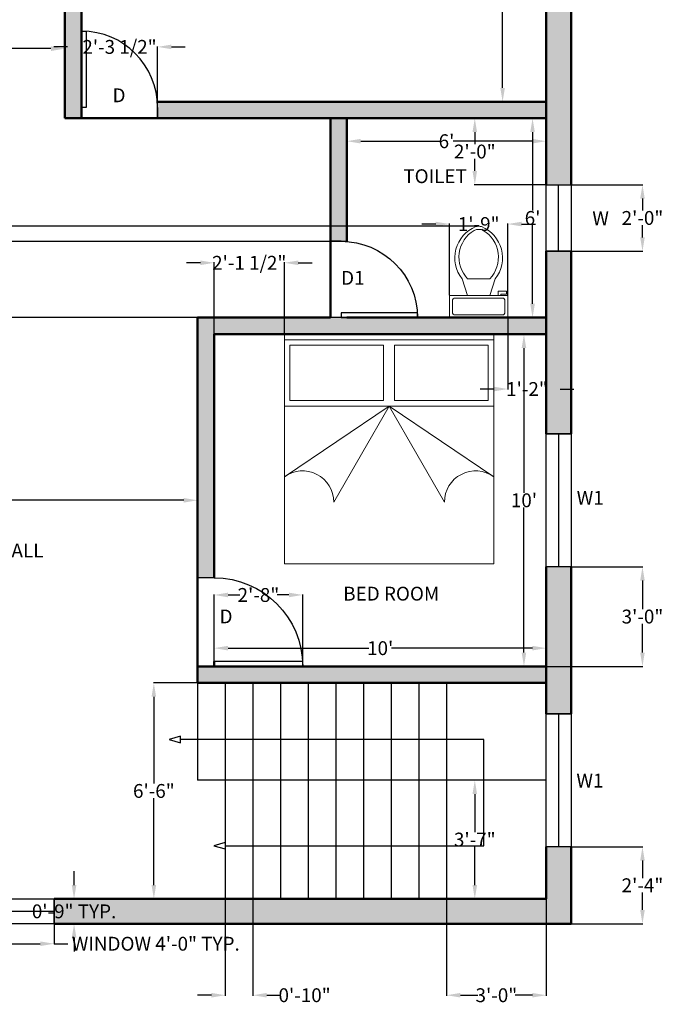
# Model space of a CAD drawing. Units: inches. Extents: x 3136 to 3620, y 13606 to 14152.
# Tile 5 of 6: x 3386 to 3618, y 13610 to 13965. Entities that reach past the tile are written whole.
import ezdxf

# ---------------------------------------------------------------- set-up
doc = ezdxf.new("R2010")
doc.units = ezdxf.units.IN
for name, color, linetype, lineweight in [('A-ANNO-DIMS', 2, 'Continuous', 18), ('A-ANNO-TEXT', 7, 'Continuous', 18), ('A-AREA-IDEN', 7, 'Continuous', 25), ('A-DOOR', 3, 'Continuous', 25), ('A-FLOR-FIXT', 9, 'Continuous', 18), ('A-FLOR-STRS', 7, 'Continuous', 25), ('A-FURN', 8, 'Continuous', 18), ('A-GLAZ', 4, 'Continuous', 25), ('A-WALL', 7, 'Continuous', 50), ('A-WALL-PATT', 174, 'Continuous', 13)]:
    doc.layers.add(name, color=color, linetype=linetype, lineweight=lineweight)
doc.styles.get("Standard").update_dxf_attribs({"font": 'arial.ttf', "height": 5})
doc.dimstyles.get("Standard").update_dxf_attribs({"dimtxt": 5, "dimasz": 5, "dimexe": 0.18, "dimexo": 0.0625, "dimgap": 0.09, "dimtad": 0, "dimtih": 1, "dimtoh": 1, "dimdec": 0, "dimzin": 0, "dimdsep": 46, "dimlunit": 3, "dimtxsty": 'Standard', "dimcen": 0.09, "dimadec": 0, "dimazin": 0, "dimtfac": 1, "dimtdec": 0, "dimtofl": 0, "dimtmove": 0, "dimatfit": 3, "dimfxl": 1, "dimtolj": 1, "dimtzin": 0, "dimarcsym": 0})

# ---------------------------------------------------------------- blocks, each defined once
blk = doc.blocks.new('*U4')
for p, q in [((0, 0), (0, -6)), ((32, 0), (32, -6))]:
    blk.add_line(p, q)
blk.add_lwpolyline([(0, 0), (0, 32), (1.75, 32), (1.75, 0)], close=True)
blk.add_arc((0, 0), 32, 0, 90)
blk = doc.blocks.new('*U5')
for p, q in [((0, 0), (0, -100)), ((700, 0), (700, -100))]:
    blk.add_line(p, q)
blk.add_lwpolyline([(0, 0), (0, 700), (43.75, 700), (43.75, 0)], close=True)
blk.add_arc((0, 0), 700, 0, 90)
blk = doc.blocks.new('*D6')
at = {"layer": 'A-ANNO-DIMS', "color": 0, "lineweight": -2, "transparency": 16777216}
for p, q in [((3575.81, 13851.84), (3567.65, 13851.84)), ((3567.83, 13846.84), (3567.83, 13794.48)), ((3567.83, 13736.84), (3567.83, 13789.2)), ((3575.81, 13731.84), (3567.65, 13731.84))]:
    blk.add_line(p, q, dxfattribs=at)
at = {"layer": 'A-ANNO-DIMS', "color": 0, "transparency": 16777216}
for points in [[(3567, 13846.84), (3568.67, 13846.84), (3567.83, 13851.84)], [(3567, 13736.84), (3568.67, 13736.84), (3567.83, 13731.84)]]:
    blk.add_solid(points, dxfattribs=at)
at = {"layer": 'Defpoints', "color": 0, "transparency": 16777216}
for p in [(3567.83, 13851.84), (3575.87, 13851.84), (3575.87, 13731.84)]:
    blk.add_point(p, dxfattribs=at)
at = {"layer": 'A-ANNO-DIMS', "color": 0, "transparency": 16777216, "insert": (3567.83, 13791.84), "char_height": 5, "attachment_point": 5}
blk.add_mtext("\\A1;10'", dxfattribs=at)
blk = doc.blocks.new('*D7')
at = {"layer": 'A-ANNO-DIMS', "color": 0, "lineweight": -2, "transparency": 16777216}
for p, q in [((3575.81, 13929.84), (3570.77, 13929.84)), ((3570.95, 13924.84), (3570.95, 13896.48)), ((3570.95, 13862.84), (3570.95, 13891.2)), ((3575.81, 13857.84), (3570.77, 13857.84))]:
    blk.add_line(p, q, dxfattribs=at)
at = {"layer": 'A-ANNO-DIMS', "color": 0, "transparency": 16777216}
for points in [[(3570.11, 13924.84), (3571.78, 13924.84), (3570.95, 13929.84)], [(3570.11, 13862.84), (3571.78, 13862.84), (3570.95, 13857.84)]]:
    blk.add_solid(points, dxfattribs=at)
at = {"layer": 'Defpoints', "color": 0, "transparency": 16777216}
for p in [(3570.95, 13929.84), (3575.87, 13929.84), (3575.87, 13857.84)]:
    blk.add_point(p, dxfattribs=at)
at = {"layer": 'A-ANNO-DIMS', "color": 0, "transparency": 16777216, "insert": (3570.95, 13893.84), "char_height": 5, "attachment_point": 5}
blk.add_mtext("\\A1;6'", dxfattribs=at)
blk = doc.blocks.new('*D8')
at = {"layer": 'A-ANNO-DIMS', "color": 0, "lineweight": -2, "transparency": 16777216}
for p, q in [((3503.87, 13929.78), (3503.87, 13921.39)), ((3575.81, 13929.78), (3575.81, 13921.39)), ((3508.87, 13921.57), (3537.44, 13921.57)), ((3570.81, 13921.57), (3542.24, 13921.57))]:
    blk.add_line(p, q, dxfattribs=at)
at = {"layer": 'A-ANNO-DIMS', "color": 0, "transparency": 16777216}
for points in [[(3508.87, 13922.41), (3508.87, 13920.74), (3503.87, 13921.57)], [(3570.81, 13922.41), (3570.81, 13920.74), (3575.81, 13921.57)]]:
    blk.add_solid(points, dxfattribs=at)
at = {"layer": 'Defpoints', "color": 0, "transparency": 16777216}
for p in [(3503.87, 13929.84), (3575.81, 13929.84), (3575.81, 13921.57)]:
    blk.add_point(p, dxfattribs=at)
at = {"layer": 'A-ANNO-DIMS', "color": 0, "transparency": 16777216, "insert": (3539.84, 13921.57), "char_height": 5, "attachment_point": 5}
blk.add_mtext("\\A1;6'", dxfattribs=at)
blk = doc.blocks.new('*D9')
at = {"layer": 'A-ANNO-DIMS', "color": 0, "lineweight": -2, "transparency": 16777216}
for p, q in [((3575.81, 14109.84), (3559.95, 14109.84)), ((3560.13, 14104.84), (3560.13, 14025.48)), ((3560.13, 13940.84), (3560.13, 14020.2)), ((3575.81, 13935.84), (3559.95, 13935.84))]:
    blk.add_line(p, q, dxfattribs=at)
at = {"layer": 'A-ANNO-DIMS', "color": 0, "transparency": 16777216}
for points in [[(3559.29, 14104.84), (3560.96, 14104.84), (3560.13, 14109.84)], [(3559.29, 13940.84), (3560.96, 13940.84), (3560.13, 13935.84)]]:
    blk.add_solid(points, dxfattribs=at)
at = {"layer": 'Defpoints', "color": 0, "transparency": 16777216}
for p in [(3560.13, 14109.84), (3575.87, 14109.84), (3575.87, 13935.84)]:
    blk.add_point(p, dxfattribs=at)
at = {"layer": 'A-ANNO-DIMS', "color": 0, "transparency": 16777216, "insert": (3560.13, 14022.84), "char_height": 5, "attachment_point": 5}
blk.add_mtext('\\A1;14\'-6"', dxfattribs=at)
blk = doc.blocks.new('*D13')
at = {"layer": 'A-ANNO-DIMS', "color": 0, "lineweight": -2, "transparency": 16777216}
for p, q in [((3233.87, 13960.47), (3233.87, 13954.82)), ((3401.87, 13960.47), (3401.87, 13954.82)), ((3238.87, 13955), (3313.77, 13955)), ((3396.87, 13955), (3321.97, 13955))]:
    blk.add_line(p, q, dxfattribs=at)
at = {"layer": 'A-ANNO-DIMS', "color": 0, "transparency": 16777216}
for points in [[(3238.87, 13955.83), (3238.87, 13954.16), (3233.87, 13955)], [(3396.87, 13955.83), (3396.87, 13954.16), (3401.87, 13955)]]:
    blk.add_solid(points, dxfattribs=at)
at = {"layer": 'Defpoints', "color": 0, "transparency": 16777216}
for p in [(3233.87, 13960.54), (3401.87, 13960.54), (3401.87, 13955)]:
    blk.add_point(p, dxfattribs=at)
at = {"layer": 'A-ANNO-DIMS', "color": 0, "transparency": 16777216, "insert": (3317.87, 13955), "char_height": 5, "attachment_point": 5}
blk.add_mtext("\\A1;14'", dxfattribs=at)
blk = doc.blocks.new('*D15')
at = {"layer": 'A-ANNO-DIMS', "color": 0, "lineweight": -2, "transparency": 16777216}
for p, q in [((3233.87, 13788.87), (3233.87, 13792.02)), ((3238.87, 13791.84), (3337.77, 13791.84)), ((3444.87, 13791.84), (3345.97, 13791.84)), ((3449.87, 13788.87), (3449.87, 13792.02))]:
    blk.add_line(p, q, dxfattribs=at)
at = {"layer": 'A-ANNO-DIMS', "color": 0, "transparency": 16777216}
for points in [[(3238.87, 13792.67), (3238.87, 13791.01), (3233.87, 13791.84)], [(3444.87, 13792.67), (3444.87, 13791.01), (3449.87, 13791.84)]]:
    blk.add_solid(points, dxfattribs=at)
at = {"layer": 'Defpoints', "color": 0, "transparency": 16777216}
for p in [(3449.87, 13791.84), (3233.87, 13788.8), (3449.87, 13788.8)]:
    blk.add_point(p, dxfattribs=at)
at = {"layer": 'A-ANNO-DIMS', "color": 0, "transparency": 16777216, "insert": (3341.87, 13791.84), "char_height": 5, "attachment_point": 5}
blk.add_mtext("\\A1;18'", dxfattribs=at)
blk = doc.blocks.new('*U18')
for p, q in [((241.3, -152.4), (241.3, -50.8)), ((-254, -215.9), (-203.2, -215.9)), ((-254, -241.3), (-254, -215.9)), ((-177.8, -241.3), (-254, -241.3)), ((-203.2, -215.9), (-203.2, -203.2)), ((-177.8, -203.2), (-177.8, -241.3)), ((-101.6, -203.2), (-152.4, -355.6)), ((101.6, -203.2), (152.4, -355.6)), ((101.6, -355.6), (-101.6, -355.6))]:
    blk.add_line(p, q)
blk.add_lwpolyline([(266.7, -203.2), (266.7, 0), (-266.7, 0), (-266.7, -203.2)], close=True)
for points in [[(-241.3, -50.8), (-241.3, -152.4)], [(215.9, -25.4), (-215.9, -25.4)], [(-215.9, -177.8), (215.9, -177.8)]]:
    blk.add_lwpolyline(points)
for centre, radius, start, end in [((-219.1, -47.6), 22.5, 81.8699, 188.1301), ((219.1, -47.6), 22.5, 351.8699, 98.1301), ((-219.1, -155.6), 22.5, 171.8699, 278.1301), ((219.1, -155.6), 22.5, 261.8699, 8.1301), ((89.4, -548.1), 309.1, 141.46911, 247.97143), ((106.7, -554.2), 287.8, 136.36773, 238.94682), ((-89.4, -548.1), 309.1, 292.02843, 38.53071), ((-106.7, -554.2), 287.8, 301.05301, 43.63209), ((0, -708.1), 101.6, 245.73182, 294.26817), ((0, -736.6), 101.6, 254.86053, 285.13947)]:
    blk.add_arc(centre, radius, start, end)
blk = doc.blocks.new('NEW BED')
for p, q in [((-75.7, 82.92), (0, 82.92)), ((-75.7, 0), (-75.7, 82.92)), ((0, 82.92), (0, 0)), ((-75.7, 80.92), (0, 80.92)), ((-73.7, 78.92), (-39.85, 78.92)), ((-73.7, 58.92), (-73.7, 78.92)), ((-39.85, 58.92), (-39.85, 78.92)), ((-35.85, 78.92), (-2, 78.92)), ((-35.85, 58.92), (-35.85, 78.92)), ((-2, 78.92), (-2, 58.92)), ((-75.7, 56.92), (0, 56.92)), ((-37.85, 56.92), (-75.7, 31.45)), ((-73.7, 58.92), (-39.85, 58.92)), ((-37.85, 56.92), (-57.85, 22.27)), ((-37.85, 56.92), (0, 31.45)), ((-37.85, 56.92), (-17.84, 22.27)), ((-35.85, 58.92), (-2, 58.92)), ((0, 0), (-75.7, 0))]:
    blk.add_line(p, q)
for centre, start, end in [((-69.14, 22.27), 0, 125.5497), ((-6.56, 22.27), 54.4503, 180)]:
    blk.add_arc(centre, 11.28, start, end)
blk = doc.blocks.new('*D20')
at = {"layer": 'A-ANNO-DIMS', "color": 0, "lineweight": -2, "transparency": 16777216}
for p, q in [((3455.87, 13732.78), (3455.87, 13738.6)), ((3460.87, 13738.42), (3511.77, 13738.42)), ((3570.87, 13738.42), (3519.97, 13738.42)), ((3575.87, 13731.9), (3575.87, 13738.6))]:
    blk.add_line(p, q, dxfattribs=at)
at = {"layer": 'A-ANNO-DIMS', "color": 0, "transparency": 16777216}
for points in [[(3460.87, 13739.26), (3460.87, 13737.59), (3455.87, 13738.42)], [(3570.87, 13739.26), (3570.87, 13737.59), (3575.87, 13738.42)]]:
    blk.add_solid(points, dxfattribs=at)
at = {"layer": 'Defpoints', "color": 0, "transparency": 16777216}
for p in [(3455.87, 13738.42), (3455.87, 13732.71), (3575.87, 13731.84)]:
    blk.add_point(p, dxfattribs=at)
at = {"layer": 'A-ANNO-DIMS', "color": 0, "transparency": 16777216, "insert": (3515.87, 13738.42), "char_height": 5, "attachment_point": 5}
blk.add_mtext("\\A1;10'", dxfattribs=at)
blk = doc.blocks.new('WIN-48IN-GLAZING')
for p, q in [((0, 0), (0, 9)), ((48, 0), (48, 9)), ((48, 4.5), (0, 4.5))]:
    blk.add_line(p, q)
blk = doc.blocks.new('*D30')
at = {"layer": 'A-ANNO-DIMS', "color": 0, "lineweight": -2, "transparency": 16777216}
for p, q in [((3350.03, 13638.78), (3350.03, 13631.46)), ((3398.03, 13638.78), (3398.03, 13631.46)), ((3355.03, 13631.64), (3393.03, 13631.64)), ((3398.03, 13631.64), (3403.03, 13631.64))]:
    blk.add_line(p, q, dxfattribs=at)
at = {"layer": 'A-ANNO-DIMS', "color": 0, "transparency": 16777216}
for points in [[(3355.03, 13632.47), (3355.03, 13630.81), (3350.03, 13631.64)], [(3393.03, 13632.47), (3393.03, 13630.81), (3398.03, 13631.64)]]:
    blk.add_solid(points, dxfattribs=at)
at = {"layer": 'Defpoints', "color": 0, "transparency": 16777216}
for p in [(3350.03, 13638.84), (3398.03, 13638.84), (3398.03, 13631.64)]:
    blk.add_point(p, dxfattribs=at)
at = {"layer": 'A-ANNO-DIMS', "color": 0, "transparency": 16777216, "insert": (3434.76, 13631.64), "char_height": 5, "attachment_point": 5}
blk.add_mtext('\\A1;WINDOW 4\'-0" TYP.', dxfattribs=at)
blk = doc.blocks.new('*D31')
at = {"layer": 'A-ANNO-DIMS', "color": 0, "lineweight": -2, "transparency": 16777216}
for p, q in [((3405.23, 13652.84), (3405.23, 13657.84)), ((3398.1, 13647.84), (3405.41, 13647.84)), ((3398.1, 13638.84), (3405.41, 13638.84)), ((3405.23, 13633.84), (3405.23, 13628.84))]:
    blk.add_line(p, q, dxfattribs=at)
at = {"layer": 'A-ANNO-DIMS', "color": 0, "transparency": 16777216}
for points in [[(3404.4, 13652.84), (3406.07, 13652.84), (3405.23, 13647.84)], [(3404.4, 13633.84), (3406.07, 13633.84), (3405.23, 13638.84)]]:
    blk.add_solid(points, dxfattribs=at)
at = {"layer": 'Defpoints', "color": 0, "transparency": 16777216}
for p in [(3398.03, 13647.84), (3405.23, 13647.84), (3398.03, 13638.84)]:
    blk.add_point(p, dxfattribs=at)
at = {"layer": 'A-ANNO-DIMS', "color": 0, "transparency": 16777216, "insert": (3405.23, 13643.34), "char_height": 5, "attachment_point": 5}
blk.add_mtext('\\A1;0\'-9" TYP.', dxfattribs=at)
blk = doc.blocks.new('*D47')
at = {"layer": 'A-ANNO-DIMS', "color": 0, "lineweight": -2, "transparency": 16777216}
for p, q in [((3455.87, 13731.9), (3455.87, 13757.82)), ((3460.87, 13757.64), (3465.09, 13757.64)), ((3482.87, 13757.64), (3478.65, 13757.64)), ((3487.87, 13731.9), (3487.87, 13757.82))]:
    blk.add_line(p, q, dxfattribs=at)
at = {"layer": 'A-ANNO-DIMS', "color": 0, "transparency": 16777216}
for points in [[(3460.87, 13758.47), (3460.87, 13756.81), (3455.87, 13757.64)], [(3482.87, 13758.47), (3482.87, 13756.81), (3487.87, 13757.64)]]:
    blk.add_solid(points, dxfattribs=at)
at = {"layer": 'Defpoints', "color": 0, "transparency": 16777216}
for p in [(3487.87, 13757.64), (3455.87, 13731.84), (3487.87, 13731.84)]:
    blk.add_point(p, dxfattribs=at)
at = {"layer": 'A-ANNO-DIMS', "color": 0, "transparency": 16777216, "insert": (3471.87, 13757.64), "char_height": 5, "attachment_point": 5}
blk.add_mtext('\\A1;2\'-8"', dxfattribs=at)
blk = doc.blocks.new('*D48')
at = {"layer": 'A-ANNO-DIMS', "color": 0, "lineweight": -2, "transparency": 16777216}
for p, q in [((3402.87, 13955.64), (3397.87, 13955.64)), ((3407.87, 13929.9), (3407.87, 13955.82)), ((3435.43, 13929.9), (3435.43, 13955.82)), ((3440.43, 13955.64), (3445.43, 13955.64))]:
    blk.add_line(p, q, dxfattribs=at)
at = {"layer": 'A-ANNO-DIMS', "color": 0, "transparency": 16777216}
for points in [[(3402.87, 13956.47), (3402.87, 13954.81), (3407.87, 13955.64)], [(3440.43, 13956.47), (3440.43, 13954.81), (3435.43, 13955.64)]]:
    blk.add_solid(points, dxfattribs=at)
at = {"layer": 'Defpoints', "color": 0, "transparency": 16777216}
for p in [(3435.43, 13955.64), (3407.87, 13929.84), (3435.43, 13929.84)]:
    blk.add_point(p, dxfattribs=at)
at = {"layer": 'A-ANNO-DIMS', "color": 0, "transparency": 16777216, "insert": (3421.65, 13955.64), "char_height": 5, "attachment_point": 5}
blk.add_mtext('\\A1;2\'-3 1/2"', dxfattribs=at)
blk = doc.blocks.new('*D49')
at = {"layer": 'A-ANNO-DIMS', "color": 0, "lineweight": -2, "transparency": 16777216}
for p, q in [((3503.81, 13885.32), (3198.89, 13885.32)), ((3199.07, 13880.32), (3199.07, 13874.26)), ((3199.07, 13862.84), (3199.07, 13868.9)), ((3503.81, 13857.84), (3198.89, 13857.84))]:
    blk.add_line(p, q, dxfattribs=at)
at = {"layer": 'A-ANNO-DIMS', "color": 0, "transparency": 16777216}
for points in [[(3198.24, 13880.32), (3199.9, 13880.32), (3199.07, 13885.32)], [(3198.24, 13862.84), (3199.9, 13862.84), (3199.07, 13857.84)]]:
    blk.add_solid(points, dxfattribs=at)
at = {"layer": 'Defpoints', "color": 0, "transparency": 16777216}
for p in [(3199.07, 13885.32), (3503.87, 13885.32), (3503.87, 13857.84)]:
    blk.add_point(p, dxfattribs=at)
at = {"layer": 'A-ANNO-DIMS', "color": 0, "transparency": 16777216, "insert": (3199.07, 13871.58), "char_height": 5, "attachment_point": 5}
blk.add_mtext('\\A1;2\'-3 1/2"', dxfattribs=at)
blk = doc.blocks.new('*D50')
at = {"layer": 'A-ANNO-DIMS', "color": 0, "lineweight": -2, "transparency": 16777216}
for p, q in [((3584.93, 13905.84), (3610.85, 13905.84)), ((3610.67, 13900.84), (3610.67, 13896.48)), ((3610.67, 13886.84), (3610.67, 13891.2)), ((3584.93, 13881.84), (3610.85, 13881.84))]:
    blk.add_line(p, q, dxfattribs=at)
at = {"layer": 'A-ANNO-DIMS', "color": 0, "transparency": 16777216}
for points in [[(3609.84, 13900.84), (3611.5, 13900.84), (3610.67, 13905.84)], [(3609.84, 13886.84), (3611.5, 13886.84), (3610.67, 13881.84)]]:
    blk.add_solid(points, dxfattribs=at)
at = {"layer": 'Defpoints', "color": 0, "transparency": 16777216}
for p in [(3584.87, 13905.84), (3610.67, 13905.84), (3584.87, 13881.84)]:
    blk.add_point(p, dxfattribs=at)
at = {"layer": 'A-ANNO-DIMS', "color": 0, "transparency": 16777216, "insert": (3610.67, 13893.84), "char_height": 5, "attachment_point": 5}
blk.add_mtext('\\A1;2\'-0"', dxfattribs=at)
blk = doc.blocks.new('*D52')
at = {"layer": 'A-ANNO-DIMS', "color": 0, "lineweight": -2, "transparency": 16777216}
for p, q in [((3459.87, 13647.78), (3459.87, 13612.86)), ((3469.87, 13647.78), (3469.87, 13612.86)), ((3454.87, 13613.04), (3449.87, 13613.04)), ((3474.87, 13613.04), (3479.87, 13613.04))]:
    blk.add_line(p, q, dxfattribs=at)
at = {"layer": 'A-ANNO-DIMS', "color": 0, "transparency": 16777216}
for points in [[(3454.87, 13613.87), (3454.87, 13612.21), (3459.87, 13613.04)], [(3474.87, 13613.87), (3474.87, 13612.21), (3469.87, 13613.04)]]:
    blk.add_solid(points, dxfattribs=at)
at = {"layer": 'Defpoints', "color": 0, "transparency": 16777216}
for p in [(3459.87, 13647.84), (3469.87, 13647.84), (3469.87, 13613.04)]:
    blk.add_point(p, dxfattribs=at)
at = {"layer": 'A-ANNO-DIMS', "color": 0, "transparency": 16777216, "insert": (3488.55, 13613.04), "char_height": 5, "attachment_point": 5}
blk.add_mtext('\\A1;0\'-10"', dxfattribs=at)
blk = doc.blocks.new('*D53')
at = {"layer": 'A-ANNO-DIMS', "color": 0, "lineweight": -2, "transparency": 16777216}
for p, q in [((3459.81, 13725.84), (3433.89, 13725.84)), ((3434.07, 13720.84), (3434.07, 13689.48)), ((3434.07, 13652.84), (3434.07, 13684.2)), ((3459.81, 13647.84), (3433.89, 13647.84))]:
    blk.add_line(p, q, dxfattribs=at)
at = {"layer": 'A-ANNO-DIMS', "color": 0, "transparency": 16777216}
for points in [[(3433.24, 13720.84), (3434.9, 13720.84), (3434.07, 13725.84)], [(3433.24, 13652.84), (3434.9, 13652.84), (3434.07, 13647.84)]]:
    blk.add_solid(points, dxfattribs=at)
at = {"layer": 'Defpoints', "color": 0, "transparency": 16777216}
for p in [(3434.07, 13725.84), (3459.87, 13725.84), (3459.87, 13647.84)]:
    blk.add_point(p, dxfattribs=at)
at = {"layer": 'A-ANNO-DIMS', "color": 0, "transparency": 16777216, "insert": (3434.07, 13686.84), "char_height": 5, "attachment_point": 5}
blk.add_mtext('\\A1;6\'-6"', dxfattribs=at)
blk = doc.blocks.new('*D60')
at = {"layer": 'A-ANNO-DIMS', "color": 0, "lineweight": -2, "transparency": 16777216}
for p, q in [((3584.93, 13666.7), (3610.85, 13666.7)), ((3610.67, 13661.7), (3610.67, 13655.37)), ((3610.67, 13643.84), (3610.67, 13650.17)), ((3584.93, 13638.84), (3610.85, 13638.84))]:
    blk.add_line(p, q, dxfattribs=at)
at = {"layer": 'A-ANNO-DIMS', "color": 0, "transparency": 16777216}
for points in [[(3609.84, 13661.7), (3611.5, 13661.7), (3610.67, 13666.7)], [(3609.84, 13643.84), (3611.5, 13643.84), (3610.67, 13638.84)]]:
    blk.add_solid(points, dxfattribs=at)
at = {"layer": 'Defpoints', "color": 0, "transparency": 16777216}
for p in [(3584.87, 13666.7), (3610.67, 13666.7), (3584.87, 13638.84)]:
    blk.add_point(p, dxfattribs=at)
at = {"layer": 'A-ANNO-DIMS', "color": 0, "transparency": 16777216, "insert": (3610.67, 13652.77), "char_height": 5, "attachment_point": 5}
blk.add_mtext('\\A1;2\'-4"', dxfattribs=at)
blk = doc.blocks.new('*D61')
at = {"layer": 'A-ANNO-DIMS', "color": 0, "lineweight": -2, "transparency": 16777216}
for p, q in [((3584.93, 13767.84), (3610.85, 13767.84)), ((3610.67, 13762.84), (3610.67, 13752.48)), ((3610.67, 13736.84), (3610.67, 13747.19)), ((3575.93, 13731.84), (3610.85, 13731.84))]:
    blk.add_line(p, q, dxfattribs=at)
at = {"layer": 'A-ANNO-DIMS', "color": 0, "transparency": 16777216}
for points in [[(3609.84, 13762.84), (3611.5, 13762.84), (3610.67, 13767.84)], [(3609.84, 13736.84), (3611.5, 13736.84), (3610.67, 13731.84)]]:
    blk.add_solid(points, dxfattribs=at)
at = {"layer": 'Defpoints', "color": 0, "transparency": 16777216}
for p in [(3584.87, 13767.84), (3575.87, 13731.84), (3610.67, 13731.84)]:
    blk.add_point(p, dxfattribs=at)
at = {"layer": 'A-ANNO-DIMS', "color": 0, "transparency": 16777216, "insert": (3610.67, 13749.84), "char_height": 5, "attachment_point": 5}
blk.add_mtext('\\A1;3\'-0"', dxfattribs=at)
blk = doc.blocks.new('*D62')
at = {"layer": 'A-ANNO-DIMS', "color": 0, "lineweight": -2, "transparency": 16777216}
for p, q in [((3575.81, 13929.84), (3549.89, 13929.84)), ((3550.07, 13924.84), (3550.07, 13920.48)), ((3550.07, 13910.84), (3550.07, 13915.2)), ((3575.81, 13905.84), (3549.89, 13905.84))]:
    blk.add_line(p, q, dxfattribs=at)
at = {"layer": 'A-ANNO-DIMS', "color": 0, "transparency": 16777216}
for points in [[(3549.24, 13924.84), (3550.9, 13924.84), (3550.07, 13929.84)], [(3549.24, 13910.84), (3550.9, 13910.84), (3550.07, 13905.84)]]:
    blk.add_solid(points, dxfattribs=at)
at = {"layer": 'Defpoints', "color": 0, "transparency": 16777216}
for p in [(3550.07, 13929.84), (3575.87, 13929.84), (3575.87, 13905.84)]:
    blk.add_point(p, dxfattribs=at)
at = {"layer": 'A-ANNO-DIMS', "color": 0, "transparency": 16777216, "insert": (3550.07, 13917.84), "char_height": 5, "attachment_point": 5}
blk.add_mtext('\\A1;2\'-0"', dxfattribs=at)
blk = doc.blocks.new('*D69')
at = {"layer": 'A-ANNO-DIMS', "color": 0, "lineweight": -2, "transparency": 16777216}
for p, q in [((3539.87, 13647.78), (3539.87, 13612.86)), ((3575.87, 13647.78), (3575.87, 13612.86)), ((3544.87, 13613.04), (3551.14, 13613.04)), ((3570.87, 13613.04), (3564.61, 13613.04))]:
    blk.add_line(p, q, dxfattribs=at)
at = {"layer": 'A-ANNO-DIMS', "color": 0, "transparency": 16777216}
for points in [[(3544.87, 13613.87), (3544.87, 13612.21), (3539.87, 13613.04)], [(3570.87, 13613.87), (3570.87, 13612.21), (3575.87, 13613.04)]]:
    blk.add_solid(points, dxfattribs=at)
at = {"layer": 'Defpoints', "color": 0, "transparency": 16777216}
for p in [(3539.87, 13647.84), (3575.87, 13647.84), (3575.87, 13613.04)]:
    blk.add_point(p, dxfattribs=at)
at = {"layer": 'A-ANNO-DIMS', "color": 0, "transparency": 16777216, "insert": (3557.87, 13613.04), "char_height": 5, "attachment_point": 5}
blk.add_mtext('\\A1;3\'-0"', dxfattribs=at)
blk = doc.blocks.new('*D70')
at = {"layer": 'A-ANNO-DIMS', "color": 0, "lineweight": -2, "transparency": 16777216}
for p, q in [((3575.81, 13690.7), (3549.89, 13690.7)), ((3550.07, 13685.7), (3550.07, 13671.91)), ((3550.07, 13652.84), (3550.07, 13666.62)), ((3575.81, 13647.84), (3549.89, 13647.84))]:
    blk.add_line(p, q, dxfattribs=at)
at = {"layer": 'A-ANNO-DIMS', "color": 0, "transparency": 16777216}
for points in [[(3549.24, 13685.7), (3550.9, 13685.7), (3550.07, 13690.7)], [(3549.24, 13652.84), (3550.9, 13652.84), (3550.07, 13647.84)]]:
    blk.add_solid(points, dxfattribs=at)
at = {"layer": 'Defpoints', "color": 0, "transparency": 16777216}
for p in [(3550.07, 13690.7), (3575.87, 13690.7), (3575.87, 13647.84)]:
    blk.add_point(p, dxfattribs=at)
at = {"layer": 'A-ANNO-DIMS', "color": 0, "transparency": 16777216, "insert": (3550.07, 13669.27), "char_height": 5, "attachment_point": 5}
blk.add_mtext('\\A1;3\'-7"', dxfattribs=at)
blk = doc.blocks.new('*D71')
at = {"layer": 'A-ANNO-DIMS', "color": 0, "lineweight": -2, "transparency": 16777216}
for p, q in [((3535.98, 13891.64), (3530.98, 13891.64)), ((3540.98, 13865.9), (3540.98, 13891.82)), ((3561.98, 13865.9), (3561.98, 13891.82)), ((3566.98, 13891.64), (3571.98, 13891.64))]:
    blk.add_line(p, q, dxfattribs=at)
at = {"layer": 'A-ANNO-DIMS', "color": 0, "transparency": 16777216}
for points in [[(3535.98, 13892.47), (3535.98, 13890.81), (3540.98, 13891.64)], [(3566.98, 13892.47), (3566.98, 13890.81), (3561.98, 13891.64)]]:
    blk.add_solid(points, dxfattribs=at)
at = {"layer": 'Defpoints', "color": 0, "transparency": 16777216}
for p in [(3561.98, 13891.64), (3540.98, 13865.84), (3561.98, 13865.84)]:
    blk.add_point(p, dxfattribs=at)
at = {"layer": 'A-ANNO-DIMS', "color": 0, "transparency": 16777216, "insert": (3551.48, 13891.64), "char_height": 5, "attachment_point": 5}
blk.add_mtext('\\A1;1\'-9"', dxfattribs=at)
blk = doc.blocks.new('*D72')
at = {"layer": 'A-ANNO-DIMS', "color": 0, "lineweight": -2, "transparency": 16777216}
for p, q in [((3561.98, 13857.78), (3561.98, 13831.86)), ((3575.87, 13857.78), (3575.87, 13831.86)), ((3556.98, 13832.04), (3551.98, 13832.04)), ((3580.87, 13832.04), (3585.87, 13832.04))]:
    blk.add_line(p, q, dxfattribs=at)
at = {"layer": 'A-ANNO-DIMS', "color": 0, "transparency": 16777216}
for points in [[(3556.98, 13832.87), (3556.98, 13831.21), (3561.98, 13832.04)], [(3580.87, 13832.87), (3580.87, 13831.21), (3575.87, 13832.04)]]:
    blk.add_solid(points, dxfattribs=at)
at = {"layer": 'Defpoints', "color": 0, "transparency": 16777216}
for p in [(3561.98, 13857.84), (3575.87, 13857.84), (3561.98, 13832.04)]:
    blk.add_point(p, dxfattribs=at)
at = {"layer": 'A-ANNO-DIMS', "color": 0, "transparency": 16777216, "insert": (3568.93, 13832.04), "char_height": 5, "attachment_point": 5}
blk.add_mtext('\\A1;1\'-2"', dxfattribs=at)
blk = doc.blocks.new('*D73')
at = {"layer": 'A-ANNO-DIMS', "color": 0, "lineweight": -2, "transparency": 16777216}
for p, q in [((3551.42, 13890.84), (3198.89, 13890.84)), ((3199.07, 13885.84), (3199.07, 13876.98)), ((3199.07, 13862.84), (3199.07, 13871.7)), ((3540.92, 13857.84), (3198.89, 13857.84))]:
    blk.add_line(p, q, dxfattribs=at)
at = {"layer": 'A-ANNO-DIMS', "color": 0, "transparency": 16777216}
for points in [[(3198.24, 13885.84), (3199.9, 13885.84), (3199.07, 13890.84)], [(3198.24, 13862.84), (3199.9, 13862.84), (3199.07, 13857.84)]]:
    blk.add_solid(points, dxfattribs=at)
at = {"layer": 'Defpoints', "color": 0, "transparency": 16777216}
for p in [(3551.48, 13890.84), (3199.07, 13857.84), (3540.98, 13857.84)]:
    blk.add_point(p, dxfattribs=at)
at = {"layer": 'A-ANNO-DIMS', "color": 0, "transparency": 16777216, "insert": (3199.07, 13874.34), "char_height": 5, "attachment_point": 5}
blk.add_mtext('\\A1;2\'-9"', dxfattribs=at)
blk = doc.blocks.new('*D75')
at = {"layer": 'A-ANNO-DIMS', "color": 0, "lineweight": -2, "transparency": 16777216}
for p, q in [((3450.87, 13877.64), (3445.87, 13877.64)), ((3455.87, 13851.9), (3455.87, 13877.82)), ((3481.23, 13851.9), (3481.23, 13877.82)), ((3486.23, 13877.64), (3491.23, 13877.64))]:
    blk.add_line(p, q, dxfattribs=at)
at = {"layer": 'A-ANNO-DIMS', "color": 0, "transparency": 16777216}
for points in [[(3450.87, 13878.47), (3450.87, 13876.81), (3455.87, 13877.64)], [(3486.23, 13878.47), (3486.23, 13876.81), (3481.23, 13877.64)]]:
    blk.add_solid(points, dxfattribs=at)
at = {"layer": 'Defpoints', "color": 0, "transparency": 16777216}
for p in [(3481.23, 13877.64), (3455.87, 13851.84), (3481.23, 13851.84)]:
    blk.add_point(p, dxfattribs=at)
at = {"layer": 'A-ANNO-DIMS', "color": 0, "transparency": 16777216, "insert": (3468.55, 13877.64), "char_height": 5, "attachment_point": 5}
blk.add_mtext('\\A1;2\'-1 1/2"', dxfattribs=at)

msp = doc.modelspace()

# ---------------------------------------------------------------- hatches: boundary and pattern name
at = {"layer": 'A-WALL-PATT'}
h = msp.add_hatch(color=256, dxfattribs=at)
h.dxf.hatch_style = 1
h.paths.add_polyline_path([(3584.87, 13767.84), (3575.87, 13767.84), (3575.87, 13714.7), (3584.87, 13714.7)])
h.paths.add_polyline_path([(3584.87, 13666.7), (3575.87, 13666.7), (3575.87, 13647.84), (3398.03, 13647.84), (3398.03, 13638.84), (3584.87, 13638.84)])
h.paths.add_polyline_path([(3350.03, 13647.84), (3272.91, 13647.84, -0.03225), (3273.24, 13642.78), (3273.24, 13638.84), (3350.03, 13638.84)])
h.paths.add_polyline_path([(3233.87, 13724.63), (3224.87, 13724.63), (3224.87, 13638.84), (3233.87, 13638.84), (3233.87, 13642.78), (3233.87, 13682.15)])
h.paths.add_polyline_path([(3233.87, 13893.84), (3224.87, 13893.84), (3224.87, 13760.63), (3233.87, 13760.63)])
h.paths.add_polyline_path([(3356.82, 13857.84), (3233.87, 13857.84), (3233.87, 13851.84), (3356.82, 13851.84)])
h.paths.add_polyline_path([(3233.87, 14022.84), (3224.87, 14022.84), (3224.87, 13941.84), (3233.87, 13941.84)])
h.paths.add_polyline_path([(3311.51, 13983.84), (3233.87, 13983.84), (3233.87, 13977.84), (3311.51, 13977.84)])
h.paths.add_polyline_path([(3467.87, 14118.84), (3224.87, 14118.84), (3224.87, 14070.84), (3233.87, 14070.84), (3233.87, 14081.66), (3233.87, 14109.84), (3467.87, 14109.84)])
h.paths.add_polyline_path([(3575.87, 13935.84), (3435.35, 13935.84, -0.018734), (3435.43, 13933.78), (3435.43, 13929.84), (3575.87, 13929.84)])
h.paths.add_polyline_path([(3417.35, 13932.93), (3424.89, 13932.93), (3424.89, 13943.24), (3417.35, 13943.24)], flags=9)
h.paths.add_polyline_path([(3561.82, 13786.65), (3573.42, 13786.65), (3573.42, 13796.96), (3561.82, 13796.96)], flags=9)
h.paths.add_polyline_path([(3567.12, 13888.65), (3574.84, 13888.65), (3574.84, 13898.96), (3567.12, 13898.96)], flags=9)
h.paths.add_polyline_path([(3536.01, 13916.38), (3543.73, 13916.38), (3543.73, 13926.69), (3536.01, 13926.69)], flags=9)
h.paths.add_polyline_path([(3509.85, 13733.24), (3521.46, 13733.24), (3521.46, 13743.54), (3509.85, 13743.54)], flags=9)
h.paths.add_polyline_path([(3499.97, 13866.95), (3511.39, 13866.95), (3511.39, 13877.25), (3499.97, 13877.25)], flags=9)
h.paths.add_polyline_path([(3456.03, 13744.65), (3463.57, 13744.65), (3463.57, 13754.96), (3456.03, 13754.96)], flags=9)
h = msp.add_hatch(color=256, dxfattribs=at)
h.dxf.hatch_style = 1
h.paths.add_polyline_path([(3575.87, 13857.84), (3503.87, 13857.84), (3501.81, 13857.84), (3497.87, 13857.84), (3449.87, 13857.84), (3449.87, 13763.84), (3455.87, 13763.84), (3455.87, 13851.84), (3575.87, 13851.84)])
h.paths.add_polyline_path([(3584.87, 13881.84), (3575.87, 13881.84), (3575.87, 13815.84), (3584.87, 13815.84)])
h.paths.add_polyline_path([(3575.87, 13731.84), (3455.87, 13731.84), (3449.87, 13731.84), (3449.87, 13725.84), (3575.87, 13725.84)])
h.paths.add_polyline_path([(3584.87, 14007.84), (3575.87, 14007.84), (3575.87, 13905.84), (3584.87, 13905.84)])
h.paths.add_polyline_path([(3503.87, 13929.84), (3497.87, 13929.84), (3497.87, 13885.4), (3501.81, 13885.4, -0.018734), (3503.87, 13885.32)])
h.paths.add_polyline_path([(3584.87, 14118.84), (3515.87, 14118.84), (3515.87, 14109.84), (3529.72, 14109.84), (3575.87, 14109.84), (3575.87, 14055.84), (3584.87, 14055.84)])
h.paths.add_polyline_path([(3407.87, 14109.84), (3401.87, 14109.84), (3401.87, 13929.84), (3407.87, 13929.84), (3407.87, 13933.78), (3407.87, 13961.34)])

# ---------------------------------------------------------------- linework, layer by layer
at = {"layer": 'A-FLOR-STRS'}
for p, q in [((3449.87, 13725.84), (3449.87, 13690.7)), ((3459.87, 13725.84), (3459.87, 13647.84)), ((3469.87, 13725.84), (3469.87, 13647.84)), ((3479.87, 13725.84), (3479.87, 13647.84)), ((3489.87, 13725.84), (3489.87, 13647.84)), ((3499.87, 13725.84), (3499.87, 13647.84)), ((3509.87, 13725.84), (3509.87, 13647.84)), ((3519.87, 13725.84), (3519.87, 13647.84)), ((3529.87, 13725.84), (3529.87, 13647.84)), ((3539.87, 13725.84), (3539.87, 13647.84)), ((3443.74, 13704.28), (3443.74, 13706.58)), ((3553.32, 13705.43), (3443.74, 13705.43)), ((3553.32, 13667.03), (3553.32, 13705.43)), ((3575.87, 13690.7), (3449.87, 13690.7)), ((3459.87, 13667.03), (3553.32, 13667.03))]:
    msp.add_line(p, q, dxfattribs=at)
for points in [[(3443.74, 13706.58), (3439.64, 13705.43), (3443.74, 13704.28)], [(3459.87, 13668.19), (3455.77, 13667.03), (3459.87, 13665.88)]]:
    msp.add_lwpolyline(points, dxfattribs=at)
at = {"layer": 'A-GLAZ'}
for p, q in [((3575.87, 13905.84), (3584.87, 13905.84)), ((3580.37, 13881.84), (3580.37, 13905.84)), ((3575.87, 13881.84), (3584.87, 13881.84))]:
    msp.add_line(p, q, dxfattribs=at)
for points in [[(3575.87, 13905.84), (3584.87, 13905.84), (3584.87, 13881.84), (3575.87, 13881.84)], [(3575.87, 13815.84), (3584.87, 13815.84), (3584.87, 13767.84), (3575.87, 13767.84)], [(3575.87, 13714.7), (3584.87, 13714.7), (3584.87, 13666.7), (3575.87, 13666.7)], [(3350.03, 13647.84), (3398.03, 13647.84), (3398.03, 13638.84), (3350.03, 13638.84)]]:
    msp.add_lwpolyline(points, close=True, dxfattribs=at)
at = {"layer": 'A-WALL'}
for p, q in [((3401.87, 13929.84), (3401.87, 14109.84)), ((3407.87, 13929.84), (3407.87, 14109.84)), ((3575.87, 14007.84), (3575.87, 13905.84)), ((3435.35, 13935.84), (3575.87, 13935.84)), ((3401.87, 13929.84), (3575.87, 13929.84)), ((3497.87, 13929.84), (3497.87, 13857.84)), ((3503.87, 13929.84), (3503.87, 13885.32)), ((3575.87, 13881.84), (3575.87, 13815.84)), ((3449.87, 13857.84), (3449.87, 13725.84)), ((3449.87, 13857.84), (3497.87, 13857.84)), ((3503.87, 13857.84), (3575.87, 13857.84)), ((3455.87, 13851.84), (3575.87, 13851.84)), ((3455.87, 13851.84), (3455.87, 13763.84)), ((3575.87, 13851.84), (3455.87, 13851.84)), ((3575.87, 13767.84), (3575.87, 13714.7)), ((3455.87, 13731.84), (3449.87, 13731.84)), ((3455.87, 13733.59), (3455.87, 13731.84)), ((3455.87, 13731.84), (3575.87, 13731.84)), ((3449.87, 13725.84), (3575.87, 13725.84)), ((3575.87, 13666.7), (3575.87, 13647.84)), ((3575.87, 13647.84), (3398.03, 13647.84))]:
    msp.add_line(p, q, dxfattribs=at)
for points in [[(3584.87, 14007.84), (3584.87, 13905.84)], [(3584.87, 13881.84), (3584.87, 13815.84)], [(3584.87, 13767.84), (3584.87, 13714.7)], [(3584.87, 13666.7), (3584.87, 13638.84), (3398.03, 13638.84)]]:
    msp.add_lwpolyline(points, dxfattribs=at)

# ---------------------------------------------------------------- block references
at = {"layer": 'A-DOOR', "xscale": 0.0393700787401575, "yscale": 0.0393700787401575, "zscale": 0.0393700787401575}
msp.add_blockref('*U5', (3407.87, 13933.78), dxfattribs=at)
at = {"layer": 'A-DOOR', "xscale": -0.0393700787401575, "yscale": 0.0393700787401575, "zscale": 0.0393700787401575, "rotation": 269.999999999998}
msp.add_blockref('*U5', (3501.81, 13857.84), dxfattribs=at)
at = {"layer": 'A-DOOR', "xscale": -1, "rotation": 270}
msp.add_blockref('*U4', (3455.87, 13731.84), dxfattribs=at)
at = {"layer": 'A-FLOR-FIXT', "xscale": 0.0393700787401575, "yscale": 0.0393700787401575, "zscale": 0.0393700787401575, "rotation": 180}
msp.add_blockref('*U18', (3551.48, 13857.84), dxfattribs=at)
at = {"layer": 'A-FURN'}
msp.add_blockref('NEW BED', (3556.93, 13768.92), dxfattribs=at)
at = {"layer": 'A-GLAZ'}
for p, rotation in [((3584.87, 13767.84), 90.00000000000733), ((3584.87, 13666.7), 90.00000000000419)]:
    msp.add_blockref('WIN-48IN-GLAZING', p, dxfattribs=dict(at, rotation=rotation))
msp.add_blockref('WIN-48IN-GLAZING', (3350.03, 13638.84), dxfattribs=at)

# ---------------------------------------------------------------- texts
at = {"layer": 'A-ANNO-TEXT', "char_height": 5, "attachment_point": 1}
for s, width, insert in [('D', 10.3377, (3419.14, 13940.66)), ('\\pxqc;W', 22.2613, (3584.41, 13896.23)), ('D1', 9.6446, (3501.75, 13874.7)), ('\\pxqc;W1', 22.2613, (3580.65, 13795.23)), ('D ', 7.0342, (3457.82, 13752.38)), ('\\pxqc;W1', 22.2613, (3580.55, 13693.08))]:
    msp.add_mtext_dynamic_manual_height_columns(s, width=width, gutter_width=25, heights=[0], dxfattribs=dict(at, insert=insert))
at = {"layer": 'A-AREA-IDEN', "char_height": 5, "attachment_point": 1}
for s, width, insert in [('TOILET', 26.7766, (3524.24, 13911.43)), ('LIVING HALL', 50.6869, (3354.86, 13776.18)), ('BED ROOM ', 38.4631, (3502.51, 13760.61))]:
    msp.add_mtext_dynamic_manual_height_columns(s, width=width, gutter_width=25, heights=[0], dxfattribs=dict(at, insert=insert))

# ---------------------------------------------------------------- dimensions: what is measured, and where the dimension line sits
at = {"layer": 'A-ANNO-DIMS'}
for base, p1, p2, angle, override, picture, middle in [((3560.13, 14109.84), (3575.87, 13935.84), (3575.87, 14109.84), 90, {"dimclrd": 0, "dimclre": 0, "dimclrt": 0}, '*D9', (3560.13, 14022.84)), ((3550.07, 13929.84), (3575.87, 13905.84), (3575.87, 13929.84), 90, {"dimdec": 1, "dimlfac": 1, "dimrnd": 0, "dimzin": 1, "dimdsep": 46, "dimlunit": 4, "dimfrac": 2}, '*D62', (3550.07, 13917.84)), ((3570.95, 13929.84), (3575.87, 13857.84), (3575.87, 13929.84), 90, {"dimclrd": 0, "dimclre": 0, "dimclrt": 0}, '*D7', (3570.95, 13893.84)), ((3610.67, 13905.84), (3584.87, 13881.84), (3584.87, 13905.84), 90, {"dimdec": 1, "dimlfac": 1, "dimrnd": 0, "dimzin": 1, "dimdsep": 46, "dimlunit": 4, "dimfrac": 2}, '*D50', (3610.67, 13893.84)), ((3199.07, 13857.84), (3551.48, 13890.84), (3540.98, 13857.84), 90, {"dimdec": 1, "dimlfac": 1, "dimrnd": 0, "dimzin": 1, "dimdsep": 46, "dimlunit": 4, "dimfrac": 2}, '*D73', (3199.07, 13874.34)), ((3199.07, 13885.32), (3503.87, 13857.84), (3503.87, 13885.32), 90, {"dimdec": 1, "dimlfac": 1, "dimrnd": 0, "dimzin": 1, "dimdsep": 46, "dimlunit": 4, "dimfrac": 2}, '*D49', (3199.07, 13871.58)), ((3481.23, 13877.64), (3455.87, 13851.84), (3481.23, 13851.84), 0, {"dimdec": 1, "dimlfac": 1, "dimrnd": 0, "dimzin": 1, "dimdsep": 46, "dimlunit": 4, "dimfrac": 2}, '*D75', (3468.55, 13877.64)), ((3561.98, 13832.04), (3575.87, 13857.84), (3561.98, 13857.84), 180, {"dimdec": 1, "dimlfac": 1, "dimrnd": 0, "dimzin": 1, "dimdsep": 46, "dimlunit": 4, "dimfrac": 2}, '*D72', (3568.93, 13832.04)), ((3567.83, 13851.84), (3575.87, 13731.84), (3575.87, 13851.84), 90, {"dimclrd": 0, "dimclre": 0, "dimclrt": 0}, '*D6', (3567.83, 13791.84)), ((3610.67, 13731.84), (3584.87, 13767.84), (3575.87, 13731.84), 90, {"dimdec": 1, "dimlfac": 1, "dimrnd": 0, "dimzin": 1, "dimdsep": 46, "dimlunit": 4, "dimfrac": 2}, '*D61', (3610.67, 13749.84)), ((3434.07, 13725.84), (3459.87, 13647.84), (3459.87, 13725.84), 90, {"dimdec": 1, "dimlfac": 1, "dimrnd": 0, "dimzin": 1, "dimdsep": 46, "dimlunit": 4, "dimfrac": 2}, '*D53', (3434.07, 13686.84)), ((3550.07, 13690.7), (3575.87, 13647.84), (3575.87, 13690.7), 90, {"dimdec": 1, "dimlfac": 1, "dimrnd": 0, "dimzin": 1, "dimdsep": 46, "dimlunit": 4, "dimfrac": 2}, '*D70', (3550.07, 13669.27)), ((3610.67, 13666.7), (3584.87, 13638.84), (3584.87, 13666.7), 90, {"dimdec": 1, "dimlfac": 1, "dimrnd": 0, "dimzin": 1, "dimdsep": 46, "dimlunit": 4, "dimfrac": 2}, '*D60', (3610.67, 13652.77))]:
    dim = msp.add_linear_dim(base=base, p1=p1, p2=p2, angle=angle, dimstyle='Standard', override=override, dxfattribs=at)
    dim.commit()
    dim.dimension.update_dxf_attribs({"geometry": picture, "text_midpoint": middle})
for base, p1, p2, override, picture, middle in [((3435.43, 13955.64), (3407.87, 13929.84), (3435.43, 13929.84), {"dimdec": 1, "dimlfac": 1, "dimrnd": 0, "dimzin": 1, "dimdsep": 46, "dimlunit": 4, "dimfrac": 2}, '*D48', (3421.65, 13955.64)), ((3401.87, 13955), (3233.87, 13960.54), (3401.87, 13960.54), {"dimclrd": 0, "dimclre": 0, "dimclrt": 0}, '*D13', (3317.87, 13955)), ((3575.81, 13921.57), (3503.87, 13929.84), (3575.81, 13929.84), {"dimclrd": 0, "dimclre": 0, "dimclrt": 0}, '*D8', (3539.84, 13921.57)), ((3561.98, 13891.64), (3540.98, 13865.84), (3561.98, 13865.84), {"dimdec": 1, "dimlfac": 1, "dimrnd": 0, "dimzin": 1, "dimdsep": 46, "dimlunit": 4, "dimfrac": 2}, '*D71', (3551.48, 13891.64)), ((3449.87, 13791.84), (3233.87, 13788.8), (3449.87, 13788.8), {"dimclrd": 0, "dimclre": 0, "dimclrt": 0}, '*D15', (3341.87, 13791.84)), ((3487.87, 13757.64), (3455.87, 13731.84), (3487.87, 13731.84), {"dimdec": 1, "dimlfac": 1, "dimrnd": 0, "dimzin": 1, "dimdsep": 46, "dimlunit": 4, "dimfrac": 2}, '*D47', (3471.87, 13757.64)), ((3455.87, 13738.42), (3575.87, 13731.84), (3455.87, 13732.71), {"dimclrd": 0, "dimclre": 0, "dimclrt": 0}, '*D20', (3515.87, 13738.42)), ((3469.87, 13613.04), (3459.87, 13647.84), (3469.87, 13647.84), {"dimdec": 1, "dimlfac": 1, "dimrnd": 0, "dimzin": 1, "dimdsep": 46, "dimlunit": 4, "dimfrac": 2}, '*D52', (3488.55, 13613.04)), ((3575.87, 13613.04), (3539.87, 13647.84), (3575.87, 13647.84), {"dimdec": 1, "dimlfac": 1, "dimrnd": 0, "dimzin": 1, "dimdsep": 46, "dimlunit": 4, "dimfrac": 2}, '*D69', (3557.87, 13613.04))]:
    dim = msp.add_linear_dim(base=base, p1=p1, p2=p2, dimstyle='Standard', override=override, dxfattribs=at)
    dim.commit()
    dim.dimension.update_dxf_attribs({"geometry": picture, "text_midpoint": middle})
dim = msp.add_linear_dim(base=(3405.23, 13647.84), p1=(3398.03, 13638.84), p2=(3398.03, 13647.84), angle=90, text='<> TYP.', dimstyle='Standard', override={"dimdec": 1, "dimlfac": 1, "dimrnd": 0, "dimzin": 1, "dimdsep": 46, "dimlunit": 4, "dimfrac": 2}, dxfattribs=at)
dim.commit()
dim.dimension.update_dxf_attribs({"geometry": '*D31', "text_midpoint": (3405.23, 13643.34)})
dim = msp.add_linear_dim(base=(3398.03, 13631.64), p1=(3350.03, 13638.84), p2=(3398.03, 13638.84), text='WINDOW <> TYP.', dimstyle='Standard', override={"dimdec": 1, "dimlfac": 1, "dimrnd": 0, "dimzin": 1, "dimdsep": 46, "dimlunit": 4, "dimfrac": 2}, dxfattribs=at)
dim.commit()
dim.dimension.update_dxf_attribs({"geometry": '*D30', "text_midpoint": (3434.76, 13631.64)})

doc.saveas('drawing.dxf')
